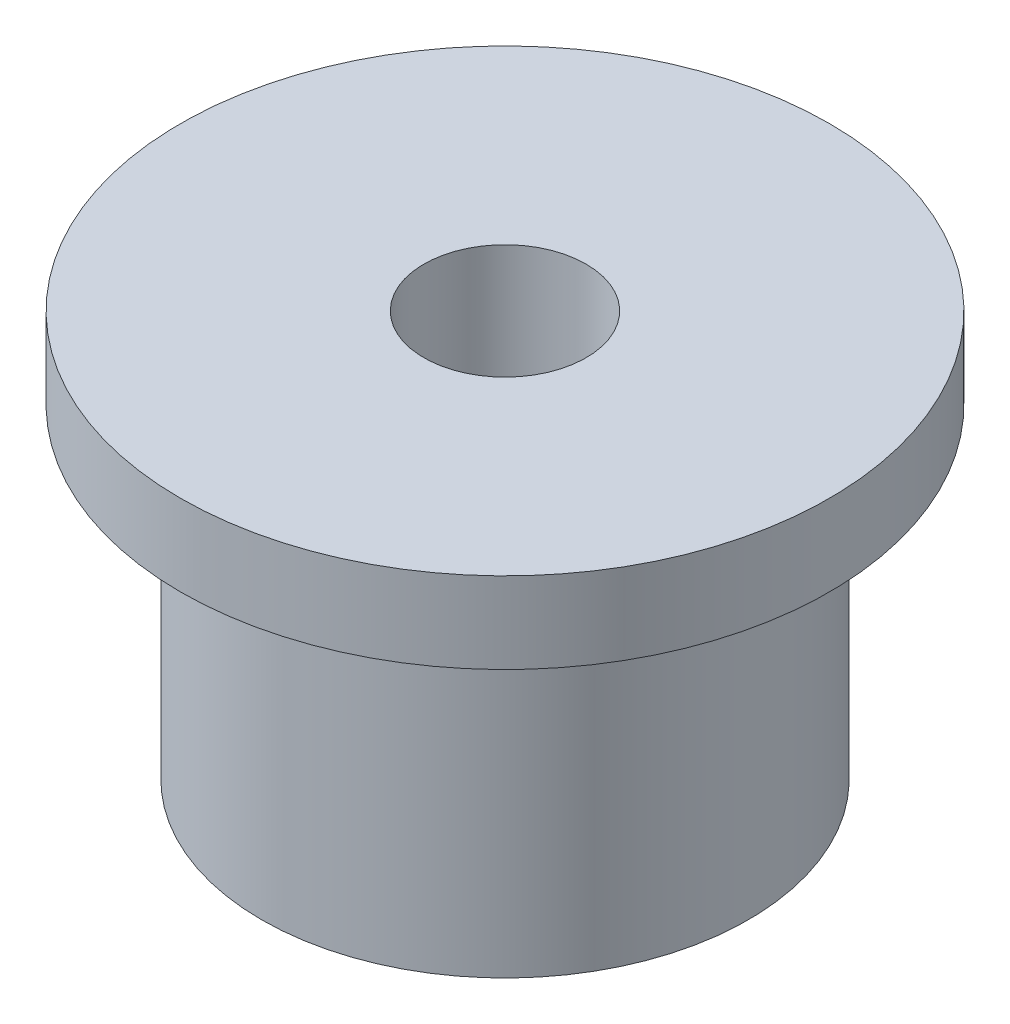
SolidWorks part; units mm, degrees
material "Plain Carbon Steel"
ref_plane "Front Plane" through (0, 0, 0) normal (0, 0, 1) x (1, 0, 0)
ref_plane "Top Plane" through (0, 0, 0) normal (0, 1, 0) x (1, 0, 0)
ref_plane "Right Plane" through (0, 0, 0) normal (1, 0, 0) x (0, 0, -1)
sketch "Bushing Half Profile" plane through (0, 0, 0) normal (0, 0, 1) x (1, 0, 0)
  line L0 (25, 0) -> (25, 125)
  line L1 (25, 125) -> (100, 125)
  line L2 (100, 125) -> (100, 100)
  line L3 (100, 100) -> (75, 100)
  line L4 (75, 100) -> (75, 0)
  line L5 (75, 0) -> (25, 0)
  line L6 (0, 0) -> (0, 189.721) construction
  dimension "D1" = 125
  dimension "D2" = 25
  dimension "D3" = 25
  dimension "D4" = 75
  dimension "D5" = 100
revolve "Flanged Bushing Revolve" add sketch "Bushing Half Profile" angle 360 about L6
